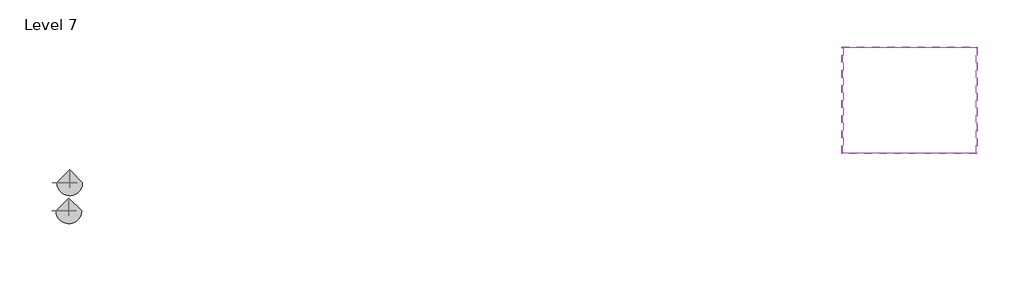
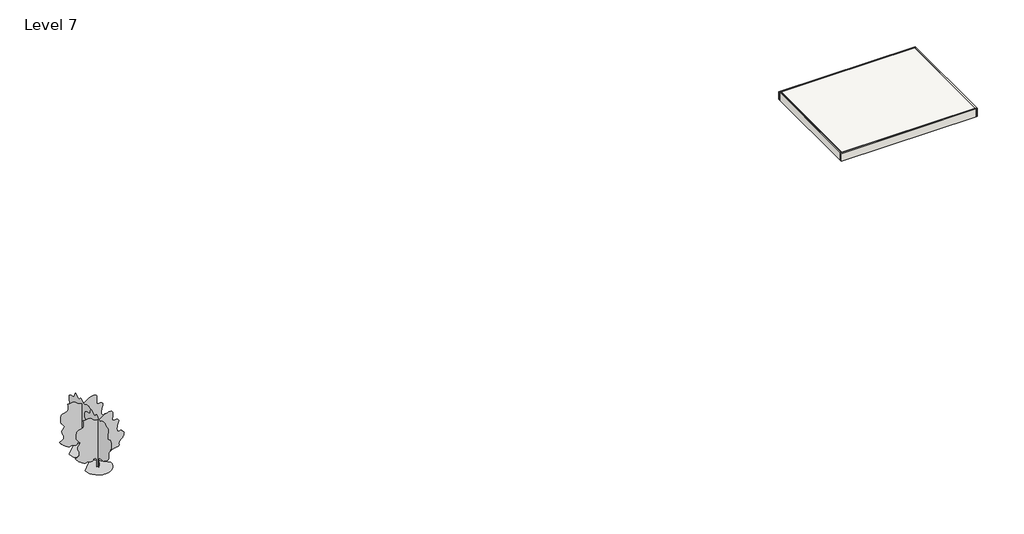
# One storey: 4 walls, 2 geographic elements, 1 slab.
"""IFC4 building model written with IfcOpenShell, lengths in millimetres."""

from ifc_helpers import new_model, si_unit, frame, origin, place, context, project, spatial, polyline, outline, extrude, faceted_brep, transform, mapped, element, save
from components import rpc_tree_deciduous_american_beech_20_b3c041c8

model = new_model("IFC4")

# Units and contexts
model_context = context("Model", 3, world=origin())
ifc_project = project(units=[si_unit("LENGTHUNIT", "METRE", prefix="MILLI")], contexts=[model_context])

# Site, building, storey
site = spatial("IfcSite", under=ifc_project)
building = spatial("IfcBuilding", under=site)
storey = spatial("IfcBuildingStorey", under=building, Name="Level 7", Elevation=18288.0)

# Geographic elements
placement = place(None, origin())
rpc_tree_deciduous_american_beech_20_shape = rpc_tree_deciduous_american_beech_20_b3c041c8(model_context)
element("IfcGeographicElement", 1, ObjectType="RPC Tree - Deciduous : American Beech - 20'", at=placement, inside=storey, context=model_context, shape_type="MappedRepresentation", body=[
    mapped(rpc_tree_deciduous_american_beech_20_shape, transform((-106763.644983, -16724.885594, 18288.0), x_axis=(1.0, 0.0, 0.0), y_axis=(0.0, 1.0, 0.0), z_axis=(0.0, 0.0, 1.0))),
])
element("IfcGeographicElement", 2, ObjectType="RPC Tree - Deciduous : American Beech - 20'", at=placement, inside=storey, context=model_context, shape_type="MappedRepresentation", body=[
    mapped(rpc_tree_deciduous_american_beech_20_shape, transform((-106690.7729387, -13525.8617616, 18288.0), x_axis=(1.0, 0.0, 0.0), y_axis=(0.0, 1.0, 0.0), z_axis=(0.0, 0.0, 1.0))),
])

# Slab
element("IfcSlab", 3, ObjectType="Generic - 12\" 5", at=placement, inside=storey, context=model_context, shape_type="SweptSolid", body=[
    extrude(outline(polyline([(-18933.7729387, 1861.2337816), (-3693.7729387, 1861.2337816), (-3693.7729387, -10178.3662184), (-18933.7729387, -10178.3662184), (-18933.7729387, 1861.2337816)])), frame((0.0, 0.0, 20116.8), z_axis=(0.0, 0.0, 1.0), x_axis=(1.0, 0.0, 0.0)), (0.0, 0.0, 1.0), 914.4),
])

# Walls
element("IfcWall", 4, ObjectType="Generic - 6\"", at=placement, inside=storey, context=model_context, shape_type="Brep", body=[
    faceted_brep([(-19009.9729387, 1785.0337816, 20116.8), (-18857.5729387, 1785.0337816, 20116.8), (-3769.9729387, 1785.0337816, 20116.8), (-3617.5729387, 1785.0337816, 20116.8), (-3617.5729387, 1785.0337816, 21031.2), (-3769.9729387, 1785.0337816, 21031.2), (-18857.5729387, 1785.0337816, 21031.2), (-19009.9729387, 1785.0337816, 21031.2), (-19009.9729387, 1937.4337816, 20116.8), (-19009.9729387, 1937.4337816, 21031.2), (-3617.5729387, 1937.4337816, 21031.2), (-3617.5729387, 1937.4337816, 20116.8)], [[[0, 1, 2, 3, 4, 5, 6, 7]], [[8, 9, 10, 11]], [[3, 2, 1, 0, 8, 11]], [[7, 6, 5, 4, 10, 9]], [[4, 3, 11, 10]], [[0, 7, 9, 8]]]),
])
element("IfcWall", 5, ObjectType="Generic - 6\"", at=placement, inside=storey, context=model_context, shape_type="Brep", body=[
    faceted_brep([(-3769.9729387, 1785.0337816, 20116.8), (-3769.9729387, -10102.1662184, 20116.8), (-3769.9729387, -10254.5662184, 20116.8), (-3769.9729387, -10254.5662184, 21031.2), (-3769.9729387, -10102.1662184, 21031.2), (-3769.9729387, 1785.0337816, 21031.2), (-3617.5729387, 1785.0337816, 20116.8), (-3617.5729387, 1785.0337816, 21031.2), (-3617.5729387, -10254.5662184, 21031.2), (-3617.5729387, -10254.5662184, 20116.8)], [[[0, 1, 2, 3, 4, 5]], [[6, 7, 8, 9]], [[2, 1, 0, 6, 9]], [[5, 4, 3, 8, 7]], [[0, 5, 7, 6]], [[3, 2, 9, 8]]]),
])
element("IfcWall", 6, ObjectType="Generic - 6\"", at=placement, inside=storey, context=model_context, shape_type="Brep", body=[
    faceted_brep([(-3769.9729387, -10102.1662184, 20116.8), (-18857.5729387, -10102.1662184, 20116.8), (-19009.9729387, -10102.1662184, 20116.8), (-19009.9729387, -10102.1662184, 21031.2), (-18857.5729387, -10102.1662184, 21031.2), (-3769.9729387, -10102.1662184, 21031.2), (-3769.9729387, -10254.5662184, 20116.8), (-3769.9729387, -10254.5662184, 21031.2), (-19009.9729387, -10254.5662184, 21031.2), (-19009.9729387, -10254.5662184, 20116.8)], [[[0, 1, 2, 3, 4, 5]], [[6, 7, 8, 9]], [[2, 1, 0, 6, 9]], [[5, 4, 3, 8, 7]], [[0, 5, 7, 6]], [[3, 2, 9, 8]]]),
])
element("IfcWall", 7, ObjectType="Generic - 6\"", at=placement, inside=storey, context=model_context, shape_type="SweptSolid", body=[
    extrude(outline(polyline([(-18857.5729387, 1785.0337816), (-18857.5729387, -10102.1662184), (-19009.9729387, -10102.1662184), (-19009.9729387, 1785.0337816), (-18857.5729387, 1785.0337816)])), frame((0.0, 0.0, 20116.8), z_axis=(0.0, 0.0, 1.0), x_axis=(1.0, 0.0, 0.0)), (0.0, 0.0, 1.0), 914.4),
])

save(model, "model.ifc")

# Revit data of these elements
# Type "RPC Tree - Deciduous : American Beech - 20'"
#   built-in parameter 1005198 = "{2, 15},{39, RPC-16-G1GQ-43Q0-7NP3-0000-ST1L-LVER-AU},{1, 0},{1, 0},{2, 13},{1, 8},{5, Color},{1, 0},{1, 0},{3, 0.8},{3, 0.8},{3, 0.8},{1, 8},{7, BBoxMin},{1, 0},{1, 0},{1, 0},{1, 0},{1, 0},{1, 8},{7, BBoxMax},{1, 0},{1, 0},{1, 0},{1, 0},{1, 0},{2, 11},{9, RPCTypeId},{1, 0},{1, 0},{39, RPC-16-G1GQ-43Q0-7NP3-0000-ST1L-LVER-AU},{1, 6},{14, RPCPlantHeight},{1, 0},{1, 0},{2, 20},{2, 11},{7, keyword},{1, 0},{1, 0},{34, :RPCs:Trees [General]:Geometry:RPC},{2, 11},{8, category},{1, 0},{1, 0},{15, Trees [General]},{2, 11},{12, LocalizedUID},{1, 0},{1, 0},{14, American Beech},{2, 14},{6, Height},{1, 0},{1, 0},{2, 20},{1, 2},{16, Cast Reflections},{1, 0},{1, 0},{1, 0},{1, 2},{12, Cast Shadows},{1, 0},{1, 0},{1, 1},{1, 2},{9, Lock View},{1, 0},{1, 0},{1, 0},{1, 4},{5, ViewC},{1, 0},{1, 0},{1, 0},{21, assetlibrary_base.fbx},{1, 5},"
#   built-in parameter 1005195 = "RPC-16-G1GQ-43Q0-7NP3-0000-ST1L-LVER-AU"
#   Type Comments = "American Beech"
#   Assembly Code = "G2050500"
#   Height = 20' - 0"
#   Default Elevation = 0
# Type "Generic - 12\" 5"
#   Assembly Code = "B1010"
#   Function = 0
#   Layers, outside or top first: 3' - 0" "Parking Stripe" (function 1)
# Type "Generic - 6\""
#   Assembly Code = "B2010"
#   Layers, outside or top first: 0' - 6" "Concrete Masonry Units" (function 1)
# Elements 1, 2 (IfcGeographicElement, "RPC Tree - Deciduous : American Beech - 20'")
#   Phase Created = New Construction
# Element 3 (IfcSlab, "Generic - 12\" 5")
#   built-in parameter 1001955 = 3.14159 (stored number, unit not read)
#   Height Offset From Level = 9' - 0"
#   Phase Created = New Construction
#   Materials on its faces: "Parking Stripe"
# Elements 4, 5, 6, 7 (IfcWall, "Generic - 6\"")
#   built-in parameter 1001111 = 6' - 0"
#   Top Offset = 0' - 0"
#   Base Offset = 6' - 0"
#   Unconnected Height = 3' - 0"
#   wall height = 3' - 0"
#   Phase Created = New Construction
#   Base Constraint = Level 7
#   Materials on its faces: "Concrete Masonry Units"
# Materials
#   "Parking Stripe": class "Paint", colour RGB 250 250 91, transparency 0, Cost = 0
#   "Concrete Masonry Units": class "Masonry", colour RGB 227 227 227, transparency 0, Description = "Concrete masonry units", Cost = 0
